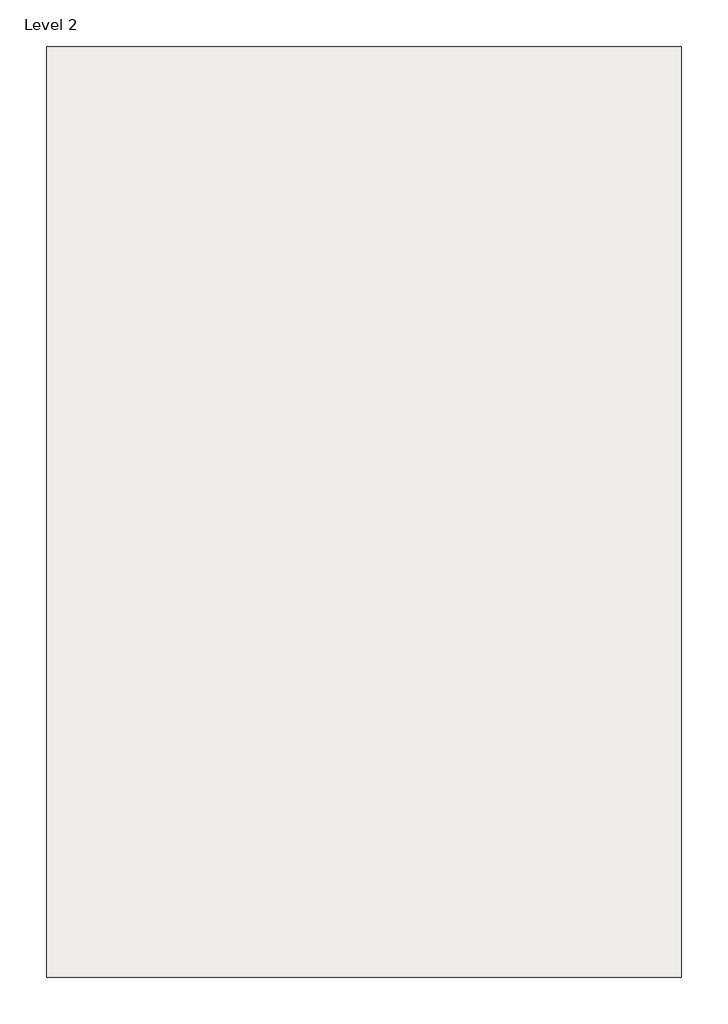
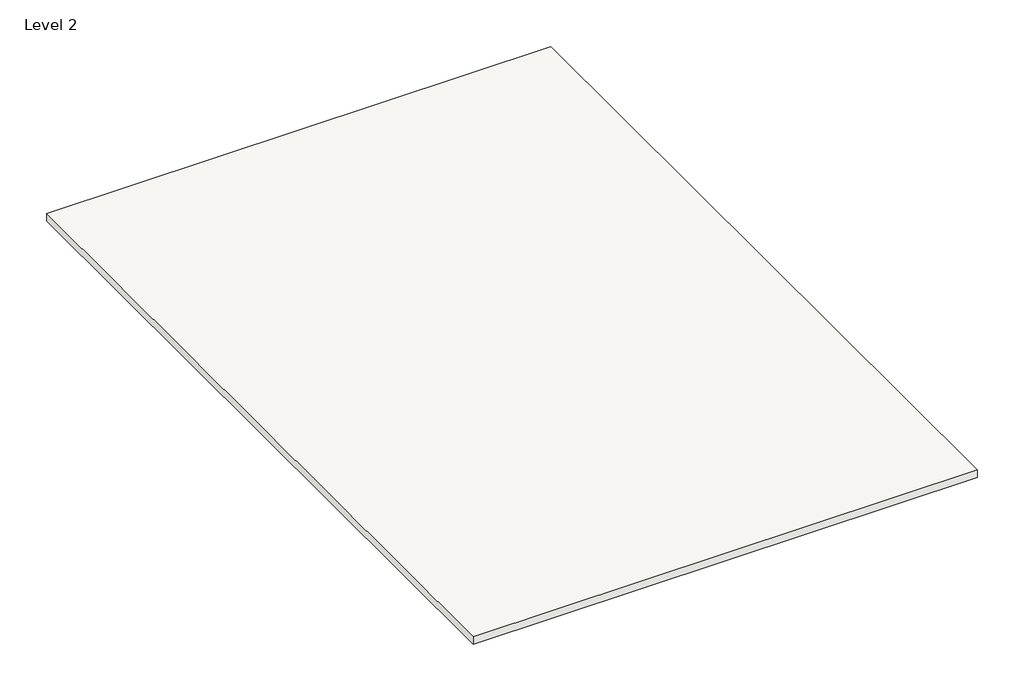
# One storey, incomplete: 1 roof.
"""IFC4 building model written with IfcOpenShell, lengths in millimetres."""

from ifc_helpers import new_model, si_unit, frame, origin, place, context, project, spatial, polyline, outline, extrude, element, save

model = new_model("IFC4")

# Units and contexts
model_context = context("Model", 3, world=origin())
ifc_project = project(units=[si_unit("LENGTHUNIT", "METRE", prefix="MILLI")], contexts=[model_context])

# Site, building, storey
site = spatial("IfcSite", under=ifc_project)
building = spatial("IfcBuilding", under=site)
storey = spatial("IfcBuildingStorey", under=building, Name="Level 2", Elevation=3048.0)

# Roof
placement = place(None, origin())
element("IfcRoof", 1, ObjectType="Generic - 12\"", at=placement, inside=storey, context=model_context, shape_type="SweptSolid", body=[
    extrude(outline(polyline([(-5991.4247832, 7671.8032079), (3647.8752168, 7671.8032079), (3647.8752168, -6450.5967921), (-5991.4247832, -6450.5967921), (-5991.4247832, 7671.8032079)])), frame((0.0, 0.0, 3048.0), z_axis=(0.0, 0.0, 1.0), x_axis=(1.0, 0.0, 0.0)), (0.0, 0.0, 1.0), 152.4),
])

save(model, "model.ifc")

# Revit data of these elements
# Type "Generic - 12\""
#   Assembly Code = "B1020"
#   Layers, outside or top first: 0' - 6" no material (function 1)
# Element 1 (IfcRoof, "Generic - 12\"")
#   built-in parameter 1001705 = 10.5 (stored number, unit not read)
#   built-in parameter 1001710 = 33615
#   Phase Created = New Construction
#   Materials on its faces: "Default Roof", "Carpet (1)"
# Materials
#   "Default Roof": colour RGB 88 101 114, transparency 0, Cost = 0
#   "Carpet (1)": class "Carpet", colour RGB 124 80 67, transparency 0, Description = "Interior finish", Cost = 0
